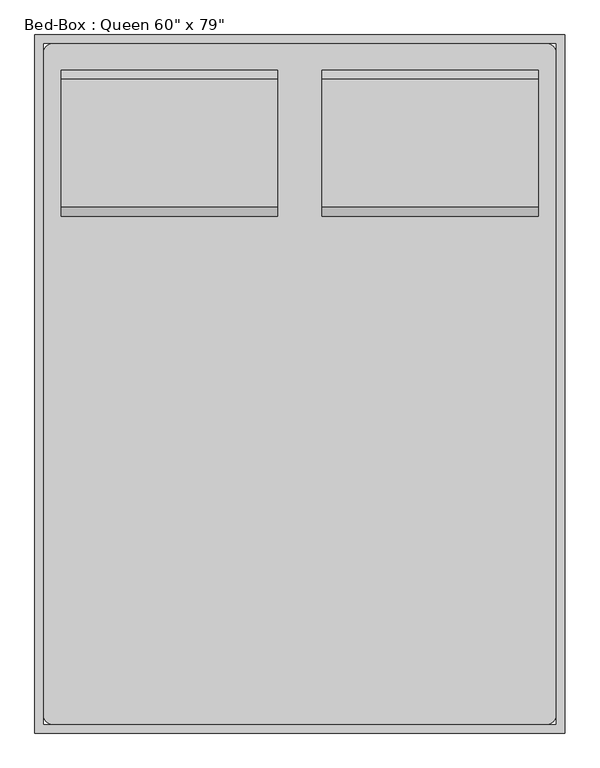
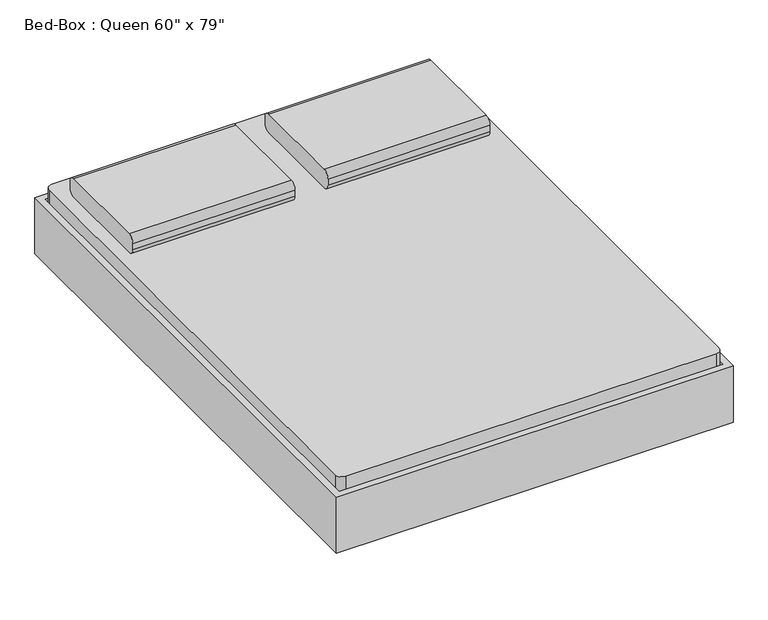
"""IFC4 building model written with IfcOpenShell, lengths in millimetres: furniture geometry."""

from ifc_helpers import new_model, si_unit, point, frame, frame_2d, origin, place, context, project, spatial, polyline, circle_curve, trimmed, segment, composite_curve, outline, extrude, source, transform, mapped, element, save
from ifc_brep_helpers import plane_surface, cylinder_surface, revolved_surface, advanced_brep


def furniture_1d2926bd(model_context):
    return source(origin(), model_context, "Body", "SolidModel", [
        extrude(outline(composite_curve([segment(polyline([(641.8704918, 406.4), (273.5704918, 406.4)]), True, "CONTINUOUS"), segment(trimmed(circle_curve(frame_2d((273.5704918, 431.8)), 25.4), [point((273.5704918, 406.4))], [point((248.1704918, 431.8))], False, "CARTESIAN"), True, "CONTINUOUS"), segment(polyline([(248.1704918, 431.8), (248.1704918, 457.2)]), True, "CONTINUOUS"), segment(trimmed(circle_curve(frame_2d((273.5704918, 457.2)), 25.4), [point((248.1704918, 457.2))], [point((273.5704918, 482.6))], False, "CARTESIAN"), True, "CONTINUOUS"), segment(polyline([(273.5704918, 482.6), (641.8704918, 482.6)]), True, "CONTINUOUS"), segment(trimmed(circle_curve(frame_2d((641.8704918, 457.2)), 25.4), [point((641.8704918, 482.6))], [point((667.2704918, 457.2))], False, "CARTESIAN"), True, "CONTINUOUS"), segment(polyline([(667.2704918, 457.2), (667.2704918, 431.8)]), True, "CONTINUOUS"), segment(trimmed(circle_curve(frame_2d((641.8704918, 431.8)), 25.4), [point((667.2704918, 431.8))], [point((641.8704918, 406.4))], False, "CARTESIAN"), True, "CONTINUOUS")], self_intersect=False)), frame((402.652459, 0.0, 0.0), z_axis=(1.0, 0.0, 0.0), x_axis=(0.0, 1.0, 0.0)), (0.0, 0.0, 1.0), 622.3),
        extrude(outline(composite_curve([segment(polyline([(641.8704918, 406.4), (273.5704918, 406.4)]), True, "CONTINUOUS"), segment(trimmed(circle_curve(frame_2d((273.5704918, 431.8)), 25.4), [point((273.5704918, 406.4))], [point((248.1704918, 431.8))], False, "CARTESIAN"), True, "CONTINUOUS"), segment(polyline([(248.1704918, 431.8), (248.1704918, 457.2)]), True, "CONTINUOUS"), segment(trimmed(circle_curve(frame_2d((273.5704918, 457.2)), 25.4), [point((248.1704918, 457.2))], [point((273.5704918, 482.6))], False, "CARTESIAN"), True, "CONTINUOUS"), segment(polyline([(273.5704918, 482.6), (641.8704918, 482.6)]), True, "CONTINUOUS"), segment(trimmed(circle_curve(frame_2d((641.8704918, 457.2)), 25.4), [point((641.8704918, 482.6))], [point((667.2704918, 457.2))], False, "CARTESIAN"), True, "CONTINUOUS"), segment(polyline([(667.2704918, 457.2), (667.2704918, 431.8)]), True, "CONTINUOUS"), segment(trimmed(circle_curve(frame_2d((641.8704918, 431.8)), 25.4), [point((667.2704918, 431.8))], [point((641.8704918, 406.4))], False, "CARTESIAN"), True, "CONTINUOUS")], self_intersect=False)), frame((-346.647541, 0.0, 0.0), z_axis=(1.0, 0.0, 0.0), x_axis=(0.0, 1.0, 0.0)), (0.0, 0.0, 1.0), 622.3),
        advanced_brep(
        [(-397.1231784, 514.8704918, 177.8), (-397.1231784, 438.6704918, 177.8), (-397.1231784, 438.6704918, 196.85), (-397.1231784, 514.8704918, 196.85), (-346.3231784, 514.8704918, 177.8), (-346.3231784, 438.6704918, 177.8), (-334.1869899, 438.6704918, 196.85), (-334.1869899, 514.8704918, 196.85), (-270.2523099, 514.8704918, 14.6654962), (-270.2523099, 438.6704918, 14.6654962), (-252.9871466, 438.6704918, 22.716374), (-252.9871466, 514.8704918, 22.716374), (-247.2320921, 438.6704918, 0.0), (-247.2320921, 514.8704918, 0.0), (-247.2320921, 438.6704918, 19.05), (-247.2320921, 514.8704918, 19.05), (-168.6195862, 514.8704918, 0.0), (-168.6195862, 438.6704918, 0.0), (-168.6195862, 438.6704918, 19.05), (-168.6195862, 514.8704918, 19.05), (-155.9195862, 438.6704918, 3.4029547), (-155.9195862, 514.8704918, 3.4029547), (-165.4445862, 438.6704918, 19.9007387), (-165.4445862, 514.8704918, 19.9007387), (-95.822541, 514.8704918, 38.1), (-95.822541, 438.6704918, 38.1), (-100.9269731, 438.6704918, 57.15), (-100.9269731, 514.8704918, 57.15), (774.4518216, 514.8704918, 38.1), (774.4518216, 438.6704918, 38.1), (779.5562537, 438.6704918, 57.15), (779.5562537, 514.8704918, 57.15), (834.5488669, 514.8704918, 3.4029547), (834.5488669, 438.6704918, 3.4029547), (844.0738669, 438.6704918, 19.9007387), (844.0738669, 514.8704918, 19.9007387), (847.2488669, 438.6704918, 0.0), (847.2488669, 514.8704918, 0.0), (847.2488669, 438.6704918, 19.05), (847.2488669, 514.8704918, 19.05), (925.8613728, 514.8704918, 0.0), (925.8613728, 438.6704918, 0.0), (925.8613728, 438.6704918, 19.05), (925.8613728, 514.8704918, 19.05), (948.8815906, 438.6704918, 14.6654962), (948.8815906, 514.8704918, 14.6654962), (931.6164272, 438.6704918, 22.716374), (931.6164272, 514.8704918, 22.716374), (1024.952459, 514.8704918, 177.8), (1024.952459, 438.6704918, 177.8), (1012.8162705, 438.6704918, 196.85), (1012.8162705, 514.8704918, 196.85), (1075.752459, 514.8704918, 177.8), (1075.752459, 514.8704918, 196.85), (1075.752459, 438.6704918, 196.85), (1075.752459, 438.6704918, 177.8)],
        [
            (0, 1),
            (1, 2),
            (2, 3),
            (3, 0),
            (0, 4),
            (4, 5),
            (5, 1),
            (5, 6),
            (6, 2),
            (6, 7),
            (7, 3),
            (7, 4),
            (4, 8),
            (8, 9),
            (9, 5),
            (9, 10),
            (10, 6),
            (10, 11),
            (11, 7),
            (11, 8),
            (12, 9, circle_curve(frame((-247.2320921, 438.6704918, 25.4), z_axis=(0.0, 1.0, 0.0), x_axis=(-0.9063077870366486, 0.0, -0.42261826174070233)), 25.4)),
            (8, 13, circle_curve(frame((-247.2320921, 514.8704918, 25.4), z_axis=(0.0, -1.0, 0.0), x_axis=(-0.9063077870366486, 0.0, -0.42261826174070233)), 25.4)),
            (13, 12),
            (14, 10, circle_curve(frame((-247.2320921, 438.6704918, 25.4), z_axis=(0.0, 1.0, 0.0), x_axis=(-0.9063077870366486, 0.0, -0.42261826174070233)), 6.35)),
            (12, 14),
            (15, 11, circle_curve(frame((-247.2320921, 514.8704918, 25.4), z_axis=(0.0, 1.0, 0.0), x_axis=(-0.9063077870366486, 0.0, -0.42261826174070233)), 6.35)),
            (14, 15),
            (15, 13),
            (13, 16),
            (16, 17),
            (17, 12),
            (17, 18),
            (18, 14),
            (18, 19),
            (19, 15),
            (19, 16),
            (20, 17, circle_curve(frame((-168.6195862, 438.6704918, 25.4), z_axis=(0.0, 1.0, 0.0), x_axis=(0.0, 0.0, -1.0)), 25.4)),
            (16, 21, circle_curve(frame((-168.6195862, 514.8704918, 25.4), z_axis=(0.0, -1.0, 0.0), x_axis=(0.0, 0.0, -1.0)), 25.4)),
            (21, 20),
            (22, 18, circle_curve(frame((-168.6195862, 438.6704918, 25.4), z_axis=(0.0, 1.0, 0.0), x_axis=(0.0, 0.0, -1.0)), 6.35)),
            (20, 22),
            (23, 19, circle_curve(frame((-168.6195862, 514.8704918, 25.4), z_axis=(0.0, 1.0, 0.0), x_axis=(0.0, 0.0, -1.0)), 6.35)),
            (22, 23),
            (23, 21),
            (21, 24),
            (24, 25),
            (25, 20),
            (25, 26),
            (26, 22),
            (26, 27),
            (27, 23),
            (27, 24),
            (24, 28),
            (28, 29),
            (29, 25),
            (29, 30),
            (30, 26),
            (30, 31),
            (31, 27),
            (31, 28),
            (28, 32),
            (32, 33),
            (33, 29),
            (33, 34),
            (34, 30),
            (34, 35),
            (35, 31),
            (35, 32),
            (36, 33, circle_curve(frame((847.2488669, 438.6704918, 25.4), z_axis=(0.0, 1.0, 0.0), x_axis=(-0.5000000000000463, 0.0, -0.8660254037844118)), 25.4)),
            (32, 37, circle_curve(frame((847.2488669, 514.8704918, 25.4), z_axis=(0.0, -1.0, 0.0), x_axis=(-0.5000000000000463, 0.0, -0.8660254037844118)), 25.4)),
            (37, 36),
            (38, 34, circle_curve(frame((847.2488669, 438.6704918, 25.4), z_axis=(0.0, 1.0, 0.0), x_axis=(-0.5000000000000463, 0.0, -0.8660254037844118)), 6.35)),
            (36, 38),
            (39, 35, circle_curve(frame((847.2488669, 514.8704918, 25.4), z_axis=(0.0, 1.0, 0.0), x_axis=(-0.5000000000000463, 0.0, -0.8660254037844118)), 6.35)),
            (38, 39),
            (39, 37),
            (37, 40),
            (40, 41),
            (41, 36),
            (41, 42),
            (42, 38),
            (42, 43),
            (43, 39),
            (43, 40),
            (44, 41, circle_curve(frame((925.8613728, 438.6704918, 25.4), z_axis=(0.0, 1.0, 0.0), x_axis=(0.0, 0.0, -1.0)), 25.4)),
            (40, 45, circle_curve(frame((925.8613728, 514.8704918, 25.4), z_axis=(0.0, -1.0, 0.0), x_axis=(0.0, 0.0, -1.0)), 25.4)),
            (45, 44),
            (46, 42, circle_curve(frame((925.8613728, 438.6704918, 25.4), z_axis=(0.0, 1.0, 0.0), x_axis=(0.0, 0.0, -1.0)), 6.35)),
            (44, 46),
            (47, 43, circle_curve(frame((925.8613728, 514.8704918, 25.4), z_axis=(0.0, 1.0, 0.0), x_axis=(0.0, 0.0, -1.0)), 6.35)),
            (46, 47),
            (47, 45),
            (45, 48),
            (48, 49),
            (49, 44),
            (49, 50),
            (50, 46),
            (50, 51),
            (51, 47),
            (51, 48),
            (52, 53),
            (53, 54),
            (54, 55),
            (55, 52),
            (48, 52),
            (55, 49),
            (54, 50),
            (53, 51),
        ],
        [
            plane_surface(frame((-397.1231784, 768.8704918, -152.9490627), z_axis=(-1.0, 0.0, 0.0), x_axis=(0.0, 1.0, 0.0))),
            plane_surface(frame((-397.1231784, 514.8704918, 177.8), z_axis=(0.0, 0.0, -1.0), x_axis=(1.0, 0.0, 0.0))),
            plane_surface(frame((-397.1231784, 438.6704918, 177.8), z_axis=(0.0, -1.0, 0.0), x_axis=(1.0, 0.0, 0.0))),
            plane_surface(frame((-397.1231784, 438.6704918, 196.85), z_axis=(0.0, 0.0, 1.0), x_axis=(1.0, 0.0, 0.0))),
            plane_surface(frame((-397.1231784, 514.8704918, 196.85), z_axis=(0.0, 1.0, 0.0), x_axis=(1.0, 0.0, 0.0))),
            plane_surface(frame((-346.3231784, 514.8704918, 177.8), z_axis=(-0.9063077870366485, 0.0, -0.4226182617407027), x_axis=(0.4226182617407027, 0.0, -0.9063077870366485))),
            plane_surface(frame((-346.3231784, 438.6704918, 177.8), z_axis=(0.0, -1.0, 0.0), x_axis=(0.4226182617407025, 0.0, -0.9063077870366486))),
            plane_surface(frame((-334.1869899, 438.6704918, 196.85), z_axis=(0.9063077870366484, 0.0, 0.4226182617407028), x_axis=(0.4226182617407028, 0.0, -0.9063077870366484))),
            plane_surface(frame((-334.1869899, 514.8704918, 196.85), z_axis=(0.0, 1.0, 0.0), x_axis=(0.42261826174070277, 0.0, -0.9063077870366485))),
            cylinder_surface(frame((-247.2320921, 768.8704918, 25.4), z_axis=(0.0, -1.0, 0.0), x_axis=(-0.9063077870366486, 0.0, -0.42261826174070233)), 25.4),
            plane_surface(frame((-247.2320921, 438.6704918, 25.4), z_axis=(0.0, -1.0, 0.0), x_axis=(-0.9063077870366486, 0.0, -0.42261826174070233))),
            revolved_surface(polyline([(-252.9871465476827, 438.6704918, 22.71637403794654), (-252.9871465476827, 514.8704918, 22.71637403794654)]), (-247.2320921, 768.8704918, 25.4), (0.0, -1.0, 0.0)),
            plane_surface(frame((-247.2320921, 514.8704918, 25.4), z_axis=(0.0, 1.0, 0.0), x_axis=(-0.9063077870366486, 0.0, -0.42261826174070233))),
            plane_surface(frame((-247.2320921, 514.8704918, 0.0), z_axis=(0.0, 0.0, -1.0), x_axis=(1.0, 0.0, 0.0))),
            plane_surface(frame((-247.2320921, 438.6704918, 0.0), z_axis=(0.0, -1.0, 0.0), x_axis=(1.0, 0.0, 0.0))),
            plane_surface(frame((-247.2320921, 438.6704918, 19.05), z_axis=(0.0, 0.0, 1.0), x_axis=(1.0, 0.0, 0.0))),
            plane_surface(frame((-247.2320921, 514.8704918, 19.05), z_axis=(0.0, 1.0, 0.0), x_axis=(1.0, 0.0, 0.0))),
            cylinder_surface(frame((-168.6195862, 768.8704918, 25.4), z_axis=(0.0, -1.0, 0.0), x_axis=(0.0, 0.0, -1.0)), 25.4),
            plane_surface(frame((-168.6195862, 438.6704918, 25.4), z_axis=(0.0, -1.0, 0.0), x_axis=(0.0, 0.0, -1.0))),
            revolved_surface(polyline([(-168.6195862, 438.6704918, 19.049999999999997), (-168.6195862, 514.8704918, 19.049999999999997)]), (-168.6195862, 768.8704918, 25.4), (0.0, -1.0, 0.0)),
            plane_surface(frame((-168.6195862, 514.8704918, 25.4), z_axis=(0.0, 1.0, 0.0), x_axis=(0.0, 0.0, -1.0))),
            plane_surface(frame((-155.9195862, 514.8704918, 3.4029547), z_axis=(0.49999999999988004, 0.0, -0.866025403784508), x_axis=(0.866025403784508, 0.0, 0.49999999999988004))),
            plane_surface(frame((-155.9195862, 438.6704918, 3.4029547), z_axis=(0.0, -1.0, 0.0), x_axis=(0.8660254037845078, 0.0, 0.49999999999988026))),
            plane_surface(frame((-165.4445862, 438.6704918, 19.9007387), z_axis=(-0.4999999999998799, 0.0, 0.866025403784508), x_axis=(0.866025403784508, 0.0, 0.4999999999998799))),
            plane_surface(frame((-165.4445862, 514.8704918, 19.9007387), z_axis=(0.0, 1.0, 0.0), x_axis=(0.8660254037845075, 0.0, 0.49999999999988076))),
            plane_surface(frame((-95.822541, 514.8704918, 38.1), z_axis=(0.0, 0.0, -1.0), x_axis=(1.0, 0.0, 0.0))),
            plane_surface(frame((-95.822541, 438.6704918, 38.1), z_axis=(0.0, -1.0, 0.0), x_axis=(1.0, 0.0, 0.0))),
            plane_surface(frame((-100.9269731, 438.6704918, 57.15), z_axis=(0.0, 0.0, 1.0), x_axis=(1.0, 0.0, 0.0))),
            plane_surface(frame((-100.9269731, 514.8704918, 57.15), z_axis=(0.0, 1.0, 0.0), x_axis=(1.0, 0.0, 0.0))),
            plane_surface(frame((774.4518216, 514.8704918, 38.1), z_axis=(-0.5000000000000455, 0.0, -0.8660254037844125), x_axis=(0.8660254037844125, 0.0, -0.5000000000000455))),
            plane_surface(frame((774.4518216, 438.6704918, 38.1), z_axis=(0.0, -1.0, 0.0), x_axis=(0.866025403784412, 0.0, -0.5000000000000463))),
            plane_surface(frame((779.5562537, 438.6704918, 57.15), z_axis=(0.5000000000000466, 0.0, 0.8660254037844117), x_axis=(0.8660254037844117, 0.0, -0.5000000000000466))),
            plane_surface(frame((779.5562537, 514.8704918, 57.15), z_axis=(0.0, 1.0, 0.0), x_axis=(0.8660254037844115, 0.0, -0.5000000000000471))),
            cylinder_surface(frame((847.2488669, 768.8704918, 25.4), z_axis=(0.0, -1.0, 0.0), x_axis=(-0.5000000000000463, 0.0, -0.8660254037844118)), 25.4),
            plane_surface(frame((847.2488669, 438.6704918, 25.4), z_axis=(0.0, -1.0000000000000002, 0.0), x_axis=(-0.5000000000000464, 0.0, -0.866025403784412))),
            revolved_surface(polyline([(844.0738668999998, 438.6704918, 19.90073868596898), (844.0738668999998, 514.8704918, 19.90073868596898)]), (847.2488669, 768.8704918, 25.4), (0.0, -1.0, 0.0)),
            plane_surface(frame((847.2488669, 514.8704918, 25.4), z_axis=(0.0, 1.0000000000000002, 0.0), x_axis=(-0.5000000000000464, 0.0, -0.866025403784412))),
            plane_surface(frame((847.2488669, 514.8704918, 0.0), z_axis=(0.0, 0.0, -1.0), x_axis=(1.0, 0.0, 0.0))),
            plane_surface(frame((847.2488669, 438.6704918, 0.0), z_axis=(0.0, -1.0, 0.0), x_axis=(1.0, 0.0, 0.0))),
            plane_surface(frame((847.2488669, 438.6704918, 19.05), z_axis=(0.0, 0.0, 1.0), x_axis=(1.0, 0.0, 0.0))),
            plane_surface(frame((847.2488669, 514.8704918, 19.05), z_axis=(0.0, 1.0, 0.0), x_axis=(1.0, 0.0, 0.0))),
            cylinder_surface(frame((925.8613728, 768.8704918, 25.4), z_axis=(0.0, -1.0, 0.0), x_axis=(0.0, 0.0, -1.0)), 25.4),
            plane_surface(frame((925.8613728, 438.6704918, 25.4), z_axis=(0.0, -1.0, 0.0), x_axis=(0.0, 0.0, -1.0))),
            revolved_surface(polyline([(925.8613728, 438.6704918, 19.049999999999997), (925.8613728, 514.8704918, 19.049999999999997)]), (925.8613728, 768.8704918, 25.4), (0.0, -1.0, 0.0)),
            plane_surface(frame((925.8613728, 514.8704918, 25.4), z_axis=(0.0, 1.0, 0.0), x_axis=(0.0, 0.0, -1.0))),
            plane_surface(frame((948.8815906, 514.8704918, 14.6654962), z_axis=(0.90630778703668, 0.0, -0.42261826174063505), x_axis=(0.42261826174063505, 0.0, 0.90630778703668))),
            plane_surface(frame((948.8815906, 438.6704918, 14.6654962), z_axis=(0.0, -1.0, 0.0), x_axis=(0.42261826174063566, 0.0, 0.9063077870366797))),
            plane_surface(frame((931.6164272, 438.6704918, 22.716374), z_axis=(-0.9063077870366801, 0.0, 0.42261826174063477), x_axis=(0.42261826174063477, 0.0, 0.9063077870366801))),
            plane_surface(frame((931.6164272, 514.8704918, 22.716374), z_axis=(0.0, 1.0, 0.0), x_axis=(0.4226182617406345, 0.0, 0.9063077870366802))),
            plane_surface(frame((1075.752459, 768.8704918, -152.9490627), z_axis=(1.0, 0.0, 0.0), x_axis=(0.0, 1.0, 0.0))),
            plane_surface(frame((1024.952459, 514.8704918, 177.8), z_axis=(0.0, 0.0, -1.0), x_axis=(1.0, 0.0, 0.0))),
            plane_surface(frame((1024.952459, 438.6704918, 177.8), z_axis=(0.0, -1.0, 0.0), x_axis=(1.0, 0.0, 0.0))),
            plane_surface(frame((1012.8162705, 438.6704918, 196.85), z_axis=(0.0, 0.0, 1.0), x_axis=(1.0, 0.0, 0.0))),
            plane_surface(frame((1012.8162705, 514.8704918, 196.85), z_axis=(0.0, 1.0, 0.0), x_axis=(1.0, 0.0, 0.0))),
        ],
        [
            (0, [[1, 2, 3, 4]]),
            (1, [[-1, 5, 6, 7]]),
            (2, [[-2, -7, 8, 9]]),
            (3, [[-3, -9, 10, 11]]),
            (4, [[-4, -11, 12, -5]]),
            (5, [[-6, 13, 14, 15]]),
            (6, [[-8, -15, 16, 17]]),
            (7, [[-10, -17, 18, 19]]),
            (8, [[-12, -19, 20, -13]]),
            (9, [[21, -14, 22, 23]]),
            (10, [[24, -16, -21, 25]]),
            (11, [[26, -18, -24, 27]]),
            (12, [[-22, -20, -26, 28]]),
            (13, [[-23, 29, 30, 31]]),
            (14, [[-25, -31, 32, 33]]),
            (15, [[-27, -33, 34, 35]]),
            (16, [[-28, -35, 36, -29]]),
            (17, [[37, -30, 38, 39]]),
            (18, [[40, -32, -37, 41]]),
            (19, [[42, -34, -40, 43]]),
            (20, [[-38, -36, -42, 44]]),
            (21, [[-39, 45, 46, 47]]),
            (22, [[-41, -47, 48, 49]]),
            (23, [[-43, -49, 50, 51]]),
            (24, [[-44, -51, 52, -45]]),
            (25, [[-46, 53, 54, 55]]),
            (26, [[-48, -55, 56, 57]]),
            (27, [[-50, -57, 58, 59]]),
            (28, [[-52, -59, 60, -53]]),
            (29, [[-54, 61, 62, 63]]),
            (30, [[-56, -63, 64, 65]]),
            (31, [[-58, -65, 66, 67]]),
            (32, [[-60, -67, 68, -61]]),
            (33, [[69, -62, 70, 71]]),
            (34, [[72, -64, -69, 73]]),
            (35, [[74, -66, -72, 75]]),
            (36, [[-70, -68, -74, 76]]),
            (37, [[-71, 77, 78, 79]]),
            (38, [[-73, -79, 80, 81]]),
            (39, [[-75, -81, 82, 83]]),
            (40, [[-76, -83, 84, -77]]),
            (41, [[85, -78, 86, 87]]),
            (42, [[88, -80, -85, 89]]),
            (43, [[90, -82, -88, 91]]),
            (44, [[-86, -84, -90, 92]]),
            (45, [[-87, 93, 94, 95]]),
            (46, [[-89, -95, 96, 97]]),
            (47, [[-91, -97, 98, 99]]),
            (48, [[-92, -99, 100, -93]]),
            (49, [[101, 102, 103, 104]]),
            (50, [[-94, 105, -104, 106]]),
            (51, [[-96, -106, -103, 107]]),
            (52, [[-98, -107, -102, 108]]),
            (53, [[-100, -108, -101, -105]]),
        ],
    ),
        extrude(outline(composite_curve([segment(polyline([(-372.047541, 743.4704918), (1050.352459, 743.4704918)]), True, "CONTINUOUS"), segment(trimmed(circle_curve(frame_2d((1050.352459, 718.0704918)), 25.4), [point((1050.352459, 743.4704918))], [point((1075.752459, 718.0704918))], False, "CARTESIAN"), True, "CONTINUOUS"), segment(polyline([(1075.752459, 718.0704918), (1075.752459, -1186.9295082)]), True, "CONTINUOUS"), segment(trimmed(circle_curve(frame_2d((1050.352459, -1186.9295082)), 25.4), [point((1075.752459, -1186.9295082))], [point((1050.352459, -1212.3295082))], False, "CARTESIAN"), True, "CONTINUOUS"), segment(polyline([(1050.352459, -1212.3295082), (-372.047541, -1212.3295082)]), True, "CONTINUOUS"), segment(trimmed(circle_curve(frame_2d((-372.047541, -1186.9295082)), 25.4), [point((-372.047541, -1212.3295082))], [point((-397.447541, -1186.9295082))], False, "CARTESIAN"), True, "CONTINUOUS"), segment(polyline([(-397.447541, -1186.9295082), (-397.447541, 718.0704918)]), True, "CONTINUOUS"), segment(trimmed(circle_curve(frame_2d((-372.047541, 718.0704918)), 25.4), [point((-397.447541, 718.0704918))], [point((-372.047541, 743.4704918))], False, "CARTESIAN"), True, "CONTINUOUS")], self_intersect=False)), frame((0.0, 0.0, 203.2), z_axis=(0.0, 0.0, 1.0), x_axis=(1.0, 0.0, 0.0)), (0.0, 0.0, 1.0), 203.2),
        advanced_brep(
        [(-397.447541, -932.9295082, 196.85), (-397.447541, -932.9295082, 177.8), (-397.447541, -1009.1295082, 177.8), (-397.447541, -1009.1295082, 196.85), (-334.5113525, -932.9295082, 196.85), (-346.647541, -932.9295082, 177.8), (-346.647541, -1009.1295082, 177.8), (-334.5113525, -1009.1295082, 196.85), (-253.3115092, -932.9295082, 22.716374), (-270.5766725, -932.9295082, 14.6654962), (-270.5766725, -1009.1295082, 14.6654962), (-253.3115092, -1009.1295082, 22.716374), (-247.5564547, -932.9295082, 0.0), (-247.5564547, -932.9295082, 19.05), (-247.5564547, -1009.1295082, 0.0), (-247.5564547, -1009.1295082, 19.05), (-168.9439489, -932.9295082, 19.05), (-168.9439489, -932.9295082, 0.0), (-168.9439489, -1009.1295082, 0.0), (-168.9439489, -1009.1295082, 19.05), (-156.2439489, -932.9295082, 3.4029547), (-165.7689489, -932.9295082, 19.9007387), (-156.2439489, -1009.1295082, 3.4029547), (-165.7689489, -1009.1295082, 19.9007387), (-101.2513357, -932.9295082, 57.15), (-96.1469036, -932.9295082, 38.1), (-96.1469036, -1009.1295082, 38.1), (-101.2513357, -1009.1295082, 57.15), (779.5562537, -932.9295082, 57.15), (774.4518216, -932.9295082, 38.1), (774.4518216, -1009.1295082, 38.1), (779.5562537, -1009.1295082, 57.15), (844.0738669, -932.9295082, 19.9007387), (834.5488669, -932.9295082, 3.4029547), (834.5488669, -1009.1295082, 3.4029547), (844.0738669, -1009.1295082, 19.9007387), (847.2488669, -932.9295082, 0.0), (847.2488669, -932.9295082, 19.05), (847.2488669, -1009.1295082, 0.0), (847.2488669, -1009.1295082, 19.05), (925.8613728, -932.9295082, 19.05), (925.8613728, -932.9295082, 0.0), (925.8613728, -1009.1295082, 0.0), (925.8613728, -1009.1295082, 19.05), (948.8815906, -932.9295082, 14.6654962), (931.6164272, -932.9295082, 22.716374), (948.8815906, -1009.1295082, 14.6654962), (931.6164272, -1009.1295082, 22.716374), (1012.8162705, -932.9295082, 196.85), (1024.952459, -932.9295082, 177.8), (1024.952459, -1009.1295082, 177.8), (1012.8162705, -1009.1295082, 196.85), (1075.752459, -932.9295082, 196.85), (1075.752459, -1009.1295082, 196.85), (1075.752459, -1009.1295082, 177.8), (1075.752459, -932.9295082, 177.8)],
        [
            (0, 1),
            (1, 2),
            (2, 3),
            (3, 0),
            (0, 4),
            (4, 5),
            (5, 1),
            (5, 6),
            (6, 2),
            (6, 7),
            (7, 3),
            (7, 4),
            (4, 8),
            (8, 9),
            (9, 5),
            (9, 10),
            (10, 6),
            (10, 11),
            (11, 7),
            (11, 8),
            (12, 9, circle_curve(frame((-247.5564547, -932.9295082, 25.4), z_axis=(0.0, 1.0, 0.0), x_axis=(-0.906307787036663, 0.0, -0.4226182617406713)), 25.4)),
            (8, 13, circle_curve(frame((-247.5564547, -932.9295082, 25.4), z_axis=(0.0, -1.0, 0.0), x_axis=(-0.906307787036663, 0.0, -0.4226182617406713)), 6.35)),
            (13, 12),
            (14, 10, circle_curve(frame((-247.5564547, -1009.1295082, 25.4), z_axis=(0.0, 1.0, 0.0), x_axis=(-0.906307787036663, 0.0, -0.4226182617406713)), 25.4)),
            (12, 14),
            (15, 11, circle_curve(frame((-247.5564547, -1009.1295082, 25.4), z_axis=(0.0, 1.0, 0.0), x_axis=(-0.906307787036663, 0.0, -0.4226182617406713)), 6.35)),
            (14, 15),
            (15, 13),
            (13, 16),
            (16, 17),
            (17, 12),
            (17, 18),
            (18, 14),
            (18, 19),
            (19, 15),
            (19, 16),
            (20, 17, circle_curve(frame((-168.9439489, -932.9295082, 25.4), z_axis=(0.0, 1.0, 0.0), x_axis=(0.0, 0.0, -1.0)), 25.4)),
            (16, 21, circle_curve(frame((-168.9439489, -932.9295082, 25.4), z_axis=(0.0, -1.0, 0.0), x_axis=(0.0, 0.0, -1.0)), 6.35)),
            (21, 20),
            (22, 18, circle_curve(frame((-168.9439489, -1009.1295082, 25.4), z_axis=(0.0, 1.0, 0.0), x_axis=(0.0, 0.0, -1.0)), 25.4)),
            (20, 22),
            (23, 19, circle_curve(frame((-168.9439489, -1009.1295082, 25.4), z_axis=(0.0, 1.0, 0.0), x_axis=(0.0, 0.0, -1.0)), 6.35)),
            (22, 23),
            (23, 21),
            (21, 24),
            (24, 25),
            (25, 20),
            (25, 26),
            (26, 22),
            (26, 27),
            (27, 23),
            (27, 24),
            (24, 28),
            (28, 29),
            (29, 25),
            (29, 30),
            (30, 26),
            (30, 31),
            (31, 27),
            (31, 28),
            (28, 32),
            (32, 33),
            (33, 29),
            (33, 34),
            (34, 30),
            (34, 35),
            (35, 31),
            (35, 32),
            (36, 33, circle_curve(frame((847.2488669, -932.9295082, 25.4), z_axis=(0.0, 1.0, 0.0), x_axis=(-0.5000000000000479, 0.0, -0.866025403784411)), 25.4)),
            (32, 37, circle_curve(frame((847.2488669, -932.9295082, 25.4), z_axis=(0.0, -1.0, 0.0), x_axis=(-0.5000000000000479, 0.0, -0.866025403784411)), 6.35)),
            (37, 36),
            (38, 34, circle_curve(frame((847.2488669, -1009.1295082, 25.4), z_axis=(0.0, 1.0, 0.0), x_axis=(-0.5000000000000479, 0.0, -0.866025403784411)), 25.4)),
            (36, 38),
            (39, 35, circle_curve(frame((847.2488669, -1009.1295082, 25.4), z_axis=(0.0, 1.0, 0.0), x_axis=(-0.5000000000000479, 0.0, -0.866025403784411)), 6.35)),
            (38, 39),
            (39, 37),
            (37, 40),
            (40, 41),
            (41, 36),
            (41, 42),
            (42, 38),
            (42, 43),
            (43, 39),
            (43, 40),
            (44, 41, circle_curve(frame((925.8613728, -932.9295082, 25.4), z_axis=(0.0, 1.0, 0.0), x_axis=(0.0, 0.0, -1.0)), 25.4)),
            (40, 45, circle_curve(frame((925.8613728, -932.9295082, 25.4), z_axis=(0.0, -1.0, 0.0), x_axis=(0.0, 0.0, -1.0)), 6.35)),
            (45, 44),
            (46, 42, circle_curve(frame((925.8613728, -1009.1295082, 25.4), z_axis=(0.0, 1.0, 0.0), x_axis=(0.0, 0.0, -1.0)), 25.4)),
            (44, 46),
            (47, 43, circle_curve(frame((925.8613728, -1009.1295082, 25.4), z_axis=(0.0, 1.0, 0.0), x_axis=(0.0, 0.0, -1.0)), 6.35)),
            (46, 47),
            (47, 45),
            (45, 48),
            (48, 49),
            (49, 44),
            (49, 50),
            (50, 46),
            (50, 51),
            (51, 47),
            (51, 48),
            (52, 53),
            (53, 54),
            (54, 55),
            (55, 52),
            (48, 52),
            (55, 49),
            (54, 50),
            (53, 51),
        ],
        [
            plane_surface(frame((-397.447541, -1237.7295082, -127.5947323), z_axis=(-1.0, 0.0, 0.0), x_axis=(0.0, 1.0, 0.0))),
            plane_surface(frame((-397.447541, -932.9295082, 196.85), z_axis=(0.0, 1.0, 0.0), x_axis=(1.0, 0.0, 0.0))),
            plane_surface(frame((-397.447541, -932.9295082, 177.8), z_axis=(0.0, 0.0, -1.0), x_axis=(1.0, 0.0, 0.0))),
            plane_surface(frame((-397.447541, -1009.1295082, 177.8), z_axis=(0.0, -1.0, 0.0), x_axis=(1.0, 0.0, 0.0))),
            plane_surface(frame((-397.447541, -1009.1295082, 196.85), z_axis=(0.0, 0.0, 1.0), x_axis=(1.0, 0.0, 0.0))),
            plane_surface(frame((-334.5113525, -932.9295082, 196.85), z_axis=(0.0, 1.0, 0.0), x_axis=(0.4226182617406707, 0.0, -0.9063077870366634))),
            plane_surface(frame((-346.647541, -932.9295082, 177.8), z_axis=(-0.9063077870366635, 0.0, -0.4226182617406707), x_axis=(0.4226182617406707, 0.0, -0.9063077870366635))),
            plane_surface(frame((-346.647541, -1009.1295082, 177.8), z_axis=(0.0, -1.0, 0.0), x_axis=(0.422618261740671, 0.0, -0.9063077870366633))),
            plane_surface(frame((-334.5113525, -1009.1295082, 196.85), z_axis=(0.9063077870366633, 0.0, 0.42261826174067113), x_axis=(0.42261826174067113, 0.0, -0.9063077870366633))),
            plane_surface(frame((-247.5564547, -932.9295082, 25.4), z_axis=(0.0, 1.0, 0.0), x_axis=(-0.906307787036663, 0.0, -0.4226182617406713))),
            cylinder_surface(frame((-247.5564547, -1237.7295082, 25.4), z_axis=(0.0, -1.0, 0.0), x_axis=(-0.906307787036663, 0.0, -0.4226182617406713)), 25.4),
            plane_surface(frame((-247.5564547, -1009.1295082, 25.4), z_axis=(0.0, -1.0, 0.0), x_axis=(-0.906307787036663, 0.0, -0.4226182617406713))),
            revolved_surface(polyline([(-253.3115091476828, -1009.1295082, 22.716374037946736), (-253.3115091476828, -932.9295082, 22.716374037946736)]), (-247.5564547, -1237.7295082, 25.4), (0.0, -1.0, 0.0)),
            plane_surface(frame((-247.5564547, -932.9295082, 19.05), z_axis=(0.0, 1.0, 0.0), x_axis=(1.0, 0.0, 0.0))),
            plane_surface(frame((-247.5564547, -932.9295082, 0.0), z_axis=(0.0, 0.0, -1.0), x_axis=(1.0, 0.0, 0.0))),
            plane_surface(frame((-247.5564547, -1009.1295082, 0.0), z_axis=(0.0, -1.0, 0.0), x_axis=(1.0, 0.0, 0.0))),
            plane_surface(frame((-247.5564547, -1009.1295082, 19.05), z_axis=(0.0, 0.0, 1.0), x_axis=(1.0, 0.0, 0.0))),
            plane_surface(frame((-168.9439489, -932.9295082, 25.4), z_axis=(0.0, 1.0, 0.0), x_axis=(0.0, 0.0, -1.0))),
            cylinder_surface(frame((-168.9439489, -1237.7295082, 25.4), z_axis=(0.0, -1.0, 0.0), x_axis=(0.0, 0.0, -1.0)), 25.4),
            plane_surface(frame((-168.9439489, -1009.1295082, 25.4), z_axis=(0.0, -1.0, 0.0), x_axis=(0.0, 0.0, -1.0))),
            revolved_surface(polyline([(-168.9439489, -1009.1295082, 19.049999999999997), (-168.9439489, -932.9295082, 19.049999999999997)]), (-168.9439489, -1237.7295082, 25.4), (0.0, -1.0, 0.0)),
            plane_surface(frame((-165.7689489, -932.9295082, 19.9007387), z_axis=(0.0, 1.0, 0.0), x_axis=(0.8660254037844788, 0.0, 0.4999999999999306))),
            plane_surface(frame((-156.2439489, -932.9295082, 3.4029547), z_axis=(0.49999999999993017, 0.0, -0.866025403784479), x_axis=(0.866025403784479, 0.0, 0.49999999999993017))),
            plane_surface(frame((-156.2439489, -1009.1295082, 3.4029547), z_axis=(0.0, -1.0, 0.0), x_axis=(0.8660254037844785, 0.0, 0.49999999999993106))),
            plane_surface(frame((-165.7689489, -1009.1295082, 19.9007387), z_axis=(-0.4999999999999309, 0.0, 0.8660254037844786), x_axis=(0.8660254037844786, 0.0, 0.4999999999999309))),
            plane_surface(frame((-101.2513357, -932.9295082, 57.15), z_axis=(0.0, 1.0, 0.0), x_axis=(1.0, 0.0, 0.0))),
            plane_surface(frame((-96.1469036, -932.9295082, 38.1), z_axis=(0.0, 0.0, -1.0), x_axis=(1.0, 0.0, 0.0))),
            plane_surface(frame((-96.1469036, -1009.1295082, 38.1), z_axis=(0.0, -1.0, 0.0), x_axis=(1.0, 0.0, 0.0))),
            plane_surface(frame((-101.2513357, -1009.1295082, 57.15), z_axis=(0.0, 0.0, 1.0), x_axis=(1.0, 0.0, 0.0))),
            plane_surface(frame((779.5562537, -932.9295082, 57.15), z_axis=(0.0, 1.0000000000000002, 0.0), x_axis=(0.8660254037844106, 0.0, -0.5000000000000487))),
            plane_surface(frame((774.4518216, -932.9295082, 38.1), z_axis=(-0.5000000000000477, 0.0, -0.8660254037844112), x_axis=(0.8660254037844112, 0.0, -0.5000000000000477))),
            plane_surface(frame((774.4518216, -1009.1295082, 38.1), z_axis=(0.0, -1.0000000000000002, 0.0), x_axis=(0.8660254037844105, 0.0, -0.500000000000049))),
            plane_surface(frame((779.5562537, -1009.1295082, 57.15), z_axis=(0.5000000000000498, 0.0, 0.8660254037844098), x_axis=(0.8660254037844098, 0.0, -0.5000000000000498))),
            plane_surface(frame((847.2488669, -932.9295082, 25.4), z_axis=(0.0, 1.0000000000000002, 0.0), x_axis=(-0.500000000000048, 0.0, -0.8660254037844111))),
            cylinder_surface(frame((847.2488669, -1237.7295082, 25.4), z_axis=(0.0, -1.0, 0.0), x_axis=(-0.5000000000000479, 0.0, -0.866025403784411)), 25.4),
            plane_surface(frame((847.2488669, -1009.1295082, 25.4), z_axis=(0.0, -1.0000000000000002, 0.0), x_axis=(-0.500000000000048, 0.0, -0.8660254037844111))),
            revolved_surface(polyline([(844.0738668999998, -1009.1295082, 19.90073868596899), (844.0738668999998, -932.9295082, 19.90073868596899)]), (847.2488669, -1237.7295082, 25.4), (0.0, -1.0, 0.0)),
            plane_surface(frame((847.2488669, -932.9295082, 19.05), z_axis=(0.0, 1.0, 0.0), x_axis=(1.0, 0.0, 0.0))),
            plane_surface(frame((847.2488669, -932.9295082, 0.0), z_axis=(0.0, 0.0, -1.0), x_axis=(1.0, 0.0, 0.0))),
            plane_surface(frame((847.2488669, -1009.1295082, 0.0), z_axis=(0.0, -1.0, 0.0), x_axis=(1.0, 0.0, 0.0))),
            plane_surface(frame((847.2488669, -1009.1295082, 19.05), z_axis=(0.0, 0.0, 1.0), x_axis=(1.0, 0.0, 0.0))),
            plane_surface(frame((925.8613728, -932.9295082, 25.4), z_axis=(0.0, 1.0, 0.0), x_axis=(0.0, 0.0, -1.0))),
            cylinder_surface(frame((925.8613728, -1237.7295082, 25.4), z_axis=(0.0, -1.0, 0.0), x_axis=(0.0, 0.0, -1.0)), 25.4),
            plane_surface(frame((925.8613728, -1009.1295082, 25.4), z_axis=(0.0, -1.0, 0.0), x_axis=(0.0, 0.0, -1.0))),
            revolved_surface(polyline([(925.8613728, -1009.1295082, 19.049999999999997), (925.8613728, -932.9295082, 19.049999999999997)]), (925.8613728, -1237.7295082, 25.4), (0.0, -1.0, 0.0)),
            plane_surface(frame((931.6164272, -932.9295082, 22.716374), z_axis=(0.0, 1.0, 0.0), x_axis=(0.4226182617405411, 0.0, 0.9063077870367238))),
            plane_surface(frame((948.8815906, -932.9295082, 14.6654962), z_axis=(0.9063077870367237, 0.0, -0.4226182617405414), x_axis=(0.4226182617405414, 0.0, 0.9063077870367237))),
            plane_surface(frame((948.8815906, -1009.1295082, 14.6654962), z_axis=(0.0, -1.0, 0.0), x_axis=(0.42261826174054123, 0.0, 0.9063077870367238))),
            plane_surface(frame((931.6164272, -1009.1295082, 22.716374), z_axis=(-0.9063077870367237, 0.0, 0.4226182617405414), x_axis=(0.4226182617405414, 0.0, 0.9063077870367237))),
            plane_surface(frame((1075.752459, -1237.7295082, -127.5947323), z_axis=(1.0, 0.0, 0.0), x_axis=(0.0, 1.0, 0.0))),
            plane_surface(frame((1012.8162705, -932.9295082, 196.85), z_axis=(0.0, 1.0, 0.0), x_axis=(1.0, 0.0, 0.0))),
            plane_surface(frame((1024.952459, -932.9295082, 177.8), z_axis=(0.0, 0.0, -1.0), x_axis=(1.0, 0.0, 0.0))),
            plane_surface(frame((1024.952459, -1009.1295082, 177.8), z_axis=(0.0, -1.0, 0.0), x_axis=(1.0, 0.0, 0.0))),
            plane_surface(frame((1012.8162705, -1009.1295082, 196.85), z_axis=(0.0, 0.0, 1.0), x_axis=(1.0, 0.0, 0.0))),
        ],
        [
            (0, [[1, 2, 3, 4]]),
            (1, [[-1, 5, 6, 7]]),
            (2, [[-2, -7, 8, 9]]),
            (3, [[-3, -9, 10, 11]]),
            (4, [[-4, -11, 12, -5]]),
            (5, [[-6, 13, 14, 15]]),
            (6, [[-8, -15, 16, 17]]),
            (7, [[-10, -17, 18, 19]]),
            (8, [[-12, -19, 20, -13]]),
            (9, [[21, -14, 22, 23]]),
            (10, [[24, -16, -21, 25]]),
            (11, [[26, -18, -24, 27]]),
            (12, [[-22, -20, -26, 28]]),
            (13, [[-23, 29, 30, 31]]),
            (14, [[-25, -31, 32, 33]]),
            (15, [[-27, -33, 34, 35]]),
            (16, [[-28, -35, 36, -29]]),
            (17, [[37, -30, 38, 39]]),
            (18, [[40, -32, -37, 41]]),
            (19, [[42, -34, -40, 43]]),
            (20, [[-38, -36, -42, 44]]),
            (21, [[-39, 45, 46, 47]]),
            (22, [[-41, -47, 48, 49]]),
            (23, [[-43, -49, 50, 51]]),
            (24, [[-44, -51, 52, -45]]),
            (25, [[-46, 53, 54, 55]]),
            (26, [[-48, -55, 56, 57]]),
            (27, [[-50, -57, 58, 59]]),
            (28, [[-52, -59, 60, -53]]),
            (29, [[-54, 61, 62, 63]]),
            (30, [[-56, -63, 64, 65]]),
            (31, [[-58, -65, 66, 67]]),
            (32, [[-60, -67, 68, -61]]),
            (33, [[69, -62, 70, 71]]),
            (34, [[72, -64, -69, 73]]),
            (35, [[74, -66, -72, 75]]),
            (36, [[-70, -68, -74, 76]]),
            (37, [[-71, 77, 78, 79]]),
            (38, [[-73, -79, 80, 81]]),
            (39, [[-75, -81, 82, 83]]),
            (40, [[-76, -83, 84, -77]]),
            (41, [[85, -78, 86, 87]]),
            (42, [[88, -80, -85, 89]]),
            (43, [[90, -82, -88, 91]]),
            (44, [[-86, -84, -90, 92]]),
            (45, [[-87, 93, 94, 95]]),
            (46, [[-89, -95, 96, 97]]),
            (47, [[-91, -97, 98, 99]]),
            (48, [[-92, -99, 100, -93]]),
            (49, [[101, 102, 103, 104]]),
            (50, [[-94, 105, -104, 106]]),
            (51, [[-96, -106, -103, 107]]),
            (52, [[-98, -107, -102, 108]]),
            (53, [[-100, -108, -101, -105]]),
        ],
    ),
        extrude(outline(polyline([(1101.152459, 768.8704918), (1101.152459, -1237.7295082), (-422.847541, -1237.7295082), (-422.847541, 768.8704918), (1101.152459, 768.8704918)]), holes=[polyline([(1075.752459, 743.4704918), (-397.447541, 743.4704918), (-397.447541, -1212.3295082), (1075.752459, -1212.3295082), (1075.752459, 743.4704918)])]), frame((0.0, 0.0, 127.0), z_axis=(0.0, 0.0, 1.0), x_axis=(1.0, 0.0, 0.0)), (0.0, 0.0, 1.0), 228.6),
    ])


if __name__ == "__main__":
    model = new_model("IFC4")
    model_context = context("Model", 3, world=origin())
    ifc_project = project(units=[si_unit("LENGTHUNIT", "METRE", prefix="MILLI")], contexts=[model_context])
    site = spatial("IfcSite", under=ifc_project)
    building = spatial("IfcBuilding", under=site)
    placement = place(None, origin())
    furniture_shape = furniture_1d2926bd(model_context)
    element("IfcFurniture", 1, ObjectType="Bed-Box : Queen 60\" x 79\"", at=placement, inside=building, context=model_context, shape_type="MappedRepresentation", body=[
        mapped(furniture_shape, transform((0.0, 0.0, 0.0), x_axis=(1.0, 0.0, 0.0), y_axis=(0.0, 1.0, 0.0), z_axis=(0.0, 0.0, 1.0))),
    ])
    save(model, "model.ifc")

# Revit data of these elements
# Type "Bed-Box : Queen 60\" x 79\""
#   Assembly Code = "E2020200"
#   Length = 6' - 7"
#   Width = 5' - 0"
#   Frame Material = Birch
#   Mattress Material = Cherry
#   Default Elevation = 0
# Element 1 (IfcFurniture, "Bed-Box : Queen 60\" x 79\"")
#   Materials on its faces: "Birch", "Cherry"
# Materials
#   "Birch": class "Wood", colour RGB 224 178 126, transparency 0, Description = "Betula Alleghaniensis", Cost = 0
#   "Cherry": class "Wood", colour RGB 226 177 128, transparency 0, Description = "Prunus Serotina", Cost = 0
